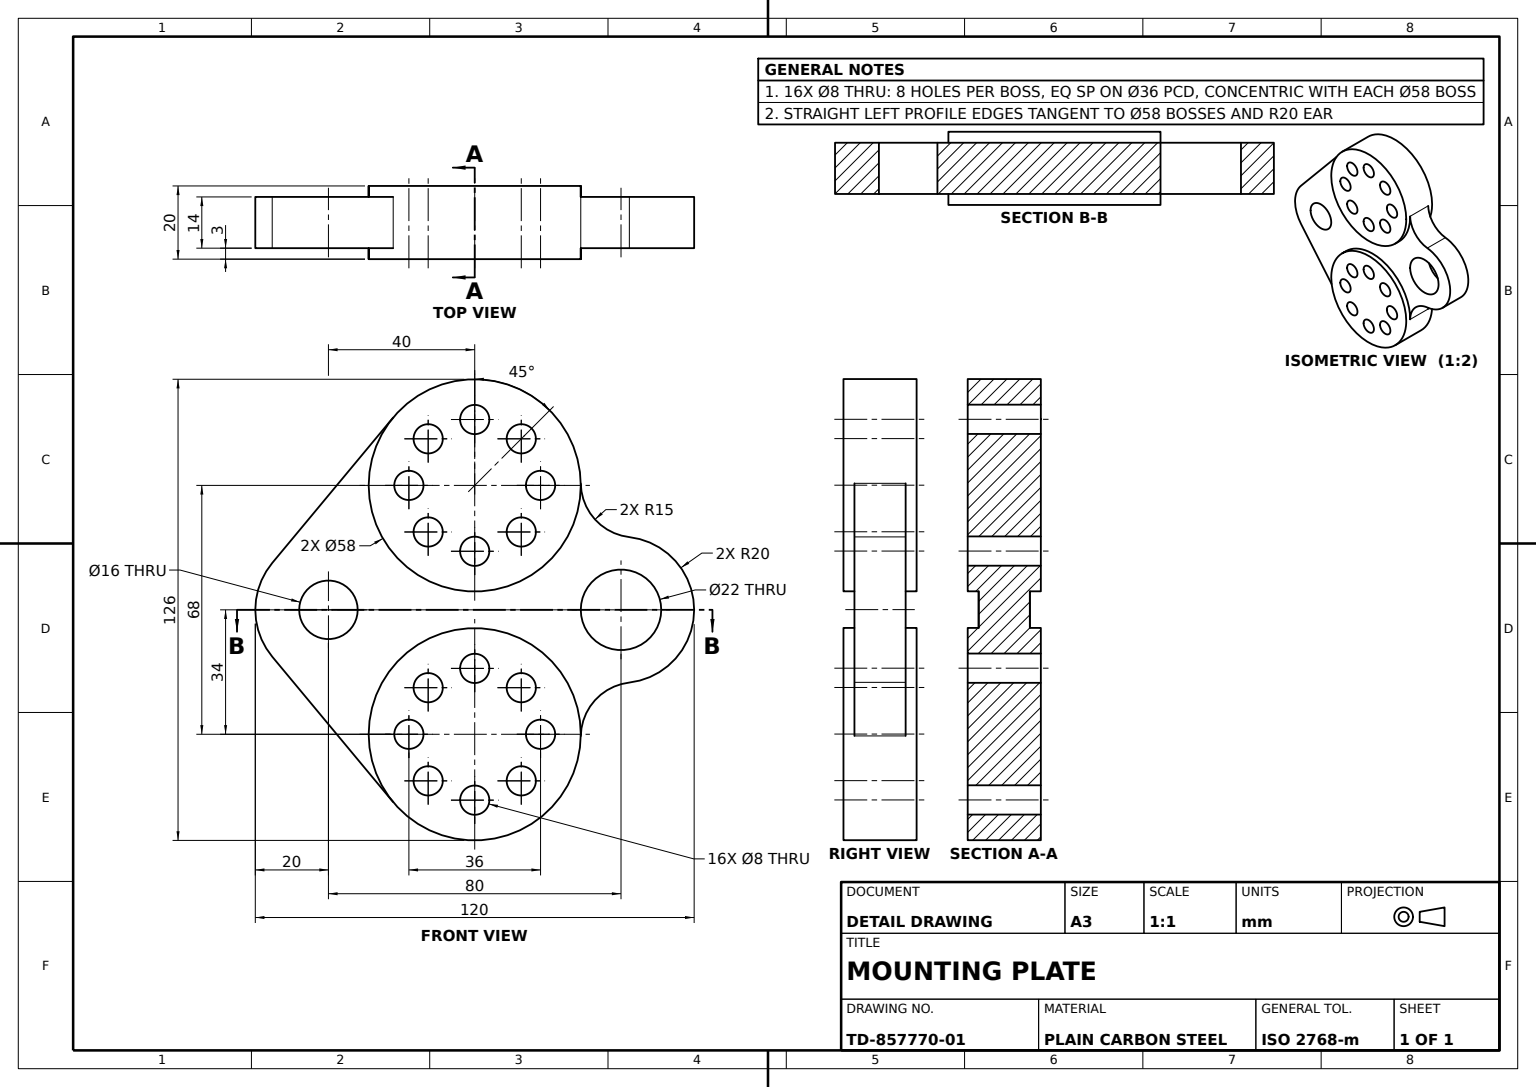
SolidWorks part; units mm, degrees
material "Plain Carbon Steel"
ref_plane "Front Plane" through (0, 0, 0) normal (0, 0, 1) x (1, 0, 0)
ref_plane "Top Plane" through (0, 0, 0) normal (0, 1, 0) x (1, 0, 0)
ref_plane "Right Plane" through (0, 0, 0) normal (1, 0, 0) x (0, 0, -1)
sketch "Plate Profile Sketch" plane through (0, 0, 0) normal (0, 0, 1) x (1, 0, 0)
  line L0 (-55.3737, -21.2074) -> (-22.2918, 18.5492)
  line L1 (-55.3737, -46.7926) -> (-22.2918, -86.5492)
  arc A0 (28.9955, 0.5085) -> (-22.2918, 18.5492) centre (0, 0) ccw
  arc A1 (-22.2918, -86.5492) -> (28.9955, -68.5085) centre (0, -68) ccw
  circle A2 centre (-40, -34) radius 8
  circle A3 centre (40, -34) radius 11
  arc A4 (-55.3737, -21.2074) -> (-55.3737, -46.7926) centre (-40, -34) ccw
  arc A5 (42.2818, -53.8694) -> (42.2818, -14.1306) centre (40, -34) ccw
  arc A6 (28.9955, -68.5085) -> (42.2818, -53.8694) centre (43.9932, -68.7715) cw
  arc A7 (28.9955, 0.5085) -> (42.2818, -14.1306) centre (43.9932, 0.7715) ccw
  dimension "D1" = 58
  dimension "D2" = 58
  dimension "D3" = 22
  dimension "D4" = 16
  dimension "D11" = 40
  dimension "D12" = 40
  dimension "D13" = 15
  dimension "D14" = 15
  dimension "D5" = 68
  dimension "D6" = 40
  dimension "D7" = 80
  dimension "D8" = 34
  dimension "D9" = 34
  dimension "D10" = 34
extrude "Connecting Plate 14mm" add sketch "Plate Profile Sketch" along normal mid plane 14
ref_plane "Plane1" through (0, 0, 0) normal (0, 0, 1) x (1, 0, 0)
sketch "Hub Bosses Sketch" plane through (0, 0, 0) normal (0, 0, 1) x (1, 0, 0)
  circle A0 centre (0, 0) radius 29
  circle A1 centre (0, -68) radius 29
  dimension "D1" = 58
  dimension "D2" = 58
  dimension "D3" = 68
extrude "Hub Bosses 20mm" add sketch "Hub Bosses Sketch" along normal mid plane 20
sketch "Bolt Circle Holes Sketch" plane through (0, 0, 10) normal (0, 0, 1) x (1, 0, 0)
  circle A2 centre (0, 18) radius 4
  circle A3 centre (12.7279, 12.7279) radius 4
  circle A4 centre (18, 0) radius 4
  circle A5 centre (12.7279, -12.7279) radius 4
  circle A6 centre (0, -18) radius 4
  circle A7 centre (-12.7279, -12.7279) radius 4
  circle A8 centre (-18, 0) radius 4
  circle A9 centre (-12.7279, 12.7279) radius 4
  circle A10 centre (0, -50) radius 4
  circle A11 centre (12.7279, -55.2721) radius 4
  circle A12 centre (18, -68) radius 4
  circle A13 centre (12.7279, -80.7279) radius 4
  circle A14 centre (0, -86) radius 4
  circle A15 centre (-12.7279, -80.7279) radius 4
  circle A16 centre (-18, -68) radius 4
  circle A17 centre (-12.7279, -55.2721) radius 4
  dimension "D1" = 12.7279
  dimension "D2" = 50
  dimension "D3" = 8
  dimension "D8" = 8
  dimension "D5" = 12.7279
  dimension "D6" = 12.7279
  dimension "D7" = 25.4558
  dimension "D10" = 86
  dimension "D11" = 18
  dimension "D12" = 12.7279
  dimension "D4" = 8
  dimension "D9" = 8
extrude "Bolt Holes 2x8xØ8" cut sketch "Bolt Circle Holes Sketch" against normal through all
